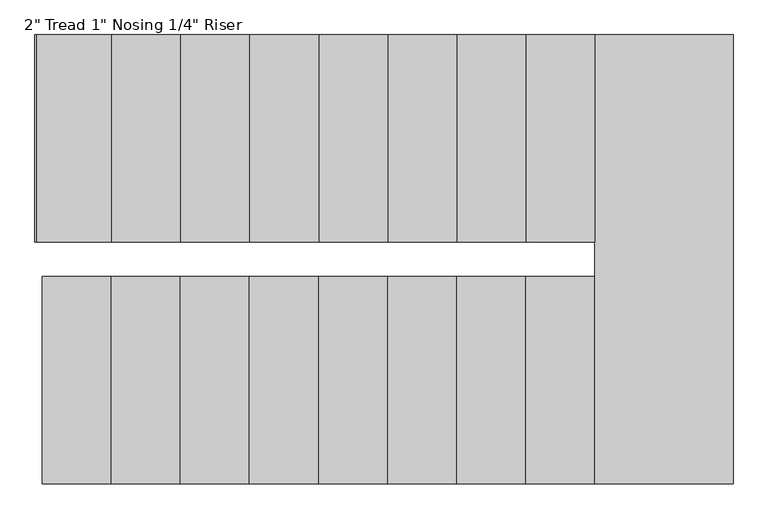
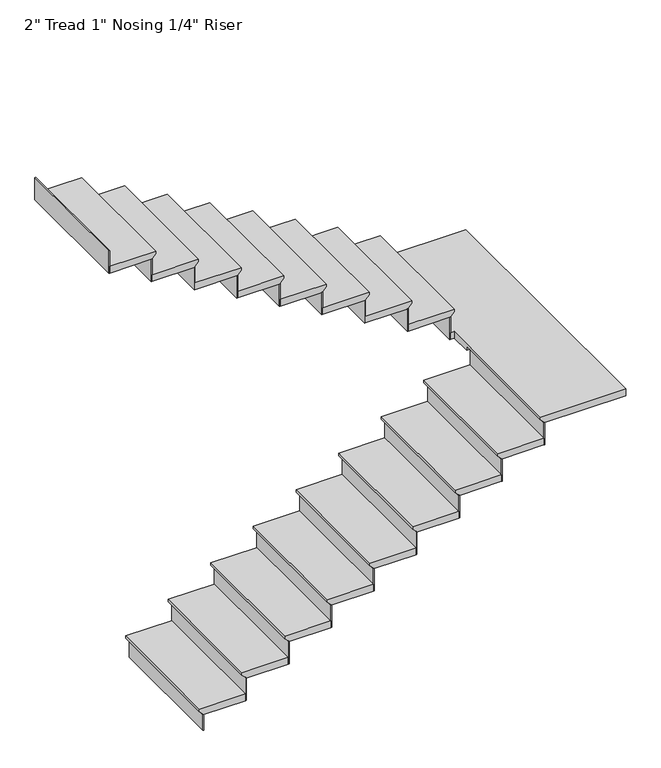
"""IFC4 building model written with IfcOpenShell, lengths in millimetres: stair flight geometry."""

from ifc_helpers import new_model, si_unit, origin, place, context, project, spatial, faceted_brep, source, transform, mapped, element, save


def stair_flight_ebc403c3(model_context):
    return source(origin(), model_context, "Body", "Brep", [
        faceted_brep([(-1197.97188, -4816.50869, 9599.0833333), (-1197.97188, -4816.50869, 9618.1333333), (-1197.97188, -3902.10869, 9618.1333333), (-1197.97188, -3902.10869, 9599.0833333), (-1172.57188, -4816.50869, 9573.6833333), (-1172.57188, -3902.10869, 9573.6833333), (-867.77188, -4816.50869, 9618.1333333), (-867.77188, -3902.10869, 9618.1333333), (-1172.57188, -3902.10869, 9567.3333333), (-867.77188, -3902.10869, 9567.3333333), (-867.77188, -4816.50869, 9567.3333333), (-1172.57188, -4816.50869, 9567.3333333)], [[[0, 1, 2, 3]], [[4, 0, 3, 5]], [[2, 1, 6, 7]], [[8, 9, 10, 11]], [[2, 7, 9, 8, 5, 3]], [[8, 11, 4, 5]], [[6, 1, 0, 4, 11, 10]], [[7, 6, 10, 9]]]),
        faceted_brep([(-1172.57188, -4816.50869, 9567.3333333), (-1172.57188, -4816.50869, 9448.8), (-1166.22188, -4816.50869, 9448.8), (-1166.22188, -4816.50869, 9567.3333333), (-1172.57188, -3902.10869, 9567.3333333), (-1166.22188, -3902.10869, 9567.3333333), (-1166.22188, -3902.10869, 9448.8), (-1172.57188, -3902.10869, 9448.8)], [[[0, 1, 2, 3]], [[4, 5, 6, 7]], [[1, 0, 4, 7]], [[2, 1, 7, 6]], [[3, 2, 6, 5]], [[0, 3, 5, 4]]]),
        faceted_brep([(-867.77188, -4816.50869, 9736.6666667), (-867.77188, -4816.50869, 9567.3333333), (-861.42188, -4816.50869, 9567.3333333), (-861.42188, -4816.50869, 9736.6666667), (-867.77188, -3902.10869, 9736.6666667), (-861.42188, -3902.10869, 9736.6666667), (-861.42188, -3902.10869, 9567.3333333), (-867.77188, -3902.10869, 9567.3333333)], [[[0, 1, 2, 3]], [[4, 5, 6, 7]], [[1, 0, 4, 7]], [[2, 1, 7, 6]], [[3, 2, 6, 5]], [[0, 3, 5, 4]]]),
        faceted_brep([(-893.17188, -3902.10869, 9787.4666667), (-893.17188, -4816.50869, 9787.4666667), (-562.97188, -4816.50869, 9787.4666667), (-562.97188, -3902.10869, 9787.4666667), (-867.77188, -3902.10869, 9736.6666667), (-562.97188, -3902.10869, 9736.6666667), (-562.97188, -4816.50869, 9736.6666667), (-867.77188, -4816.50869, 9736.6666667), (-867.77188, -3902.10869, 9743.0166667), (-893.17188, -3902.10869, 9768.4166667), (-867.77188, -4816.50869, 9743.0166667), (-893.17188, -4816.50869, 9768.4166667)], [[[0, 1, 2, 3]], [[4, 5, 6, 7]], [[0, 3, 5, 4, 8, 9]], [[4, 7, 10, 8]], [[2, 1, 11, 10, 7, 6]], [[3, 2, 6, 5]], [[11, 1, 0, 9]], [[10, 11, 9, 8]]]),
        faceted_brep([(-562.97188, -4816.50869, 9906.0), (-562.97188, -4816.50869, 9736.6666667), (-556.62188, -4816.50869, 9736.6666667), (-556.62188, -4816.50869, 9906.0), (-562.97188, -3902.10869, 9906.0), (-556.62188, -3902.10869, 9906.0), (-556.62188, -3902.10869, 9736.6666667), (-562.97188, -3902.10869, 9736.6666667)], [[[0, 1, 2, 3]], [[4, 5, 6, 7]], [[1, 0, 4, 7]], [[2, 1, 7, 6]], [[3, 2, 6, 5]], [[0, 3, 5, 4]]]),
        faceted_brep([(-588.37188, -3902.10869, 9956.8), (-588.37188, -4816.50869, 9956.8), (-258.17188, -4816.50869, 9956.8), (-258.17188, -3902.10869, 9956.8), (-562.97188, -3902.10869, 9906.0), (-258.17188, -3902.10869, 9906.0), (-258.17188, -4816.50869, 9906.0), (-562.97188, -4816.50869, 9906.0), (-562.97188, -3902.10869, 9912.35), (-588.37188, -3902.10869, 9937.75), (-562.97188, -4816.50869, 9912.35), (-588.37188, -4816.50869, 9937.75)], [[[0, 1, 2, 3]], [[4, 5, 6, 7]], [[0, 3, 5, 4, 8, 9]], [[4, 7, 10, 8]], [[2, 1, 11, 10, 7, 6]], [[3, 2, 6, 5]], [[11, 1, 0, 9]], [[10, 11, 9, 8]]]),
        faceted_brep([(-258.17188, -4816.50869, 10075.3333333), (-258.17188, -4816.50869, 9906.0), (-251.82188, -4816.50869, 9906.0), (-251.82188, -4816.50869, 10075.3333333), (-258.17188, -3902.10869, 10075.3333333), (-251.82188, -3902.10869, 10075.3333333), (-251.82188, -3902.10869, 9906.0), (-258.17188, -3902.10869, 9906.0)], [[[0, 1, 2, 3]], [[4, 5, 6, 7]], [[1, 0, 4, 7]], [[2, 1, 7, 6]], [[3, 2, 6, 5]], [[0, 3, 5, 4]]]),
        faceted_brep([(-283.57188, -3902.10869, 10126.1333333), (-283.57188, -4816.50869, 10126.1333333), (46.62812, -4816.50869, 10126.1333333), (46.62812, -3902.10869, 10126.1333333), (-258.17188, -3902.10869, 10075.3333333), (46.62812, -3902.10869, 10075.3333333), (46.62812, -4816.50869, 10075.3333333), (-258.17188, -4816.50869, 10075.3333333), (-258.17188, -3902.10869, 10081.6833333), (-283.57188, -3902.10869, 10107.0833333), (-258.17188, -4816.50869, 10081.6833333), (-283.57188, -4816.50869, 10107.0833333)], [[[0, 1, 2, 3]], [[4, 5, 6, 7]], [[0, 3, 5, 4, 8, 9]], [[4, 7, 10, 8]], [[2, 1, 11, 10, 7, 6]], [[3, 2, 6, 5]], [[11, 1, 0, 9]], [[10, 11, 9, 8]]]),
        faceted_brep([(46.62812, -4816.50869, 10244.6666667), (46.62812, -4816.50869, 10075.3333333), (52.97812, -4816.50869, 10075.3333333), (52.97812, -4816.50869, 10244.6666667), (46.62812, -3902.10869, 10244.6666667), (52.97812, -3902.10869, 10244.6666667), (52.97812, -3902.10869, 10075.3333333), (46.62812, -3902.10869, 10075.3333333)], [[[0, 1, 2, 3]], [[4, 5, 6, 7]], [[1, 0, 4, 7]], [[2, 1, 7, 6]], [[3, 2, 6, 5]], [[0, 3, 5, 4]]]),
        faceted_brep([(21.22812, -3902.10869, 10295.4666667), (21.22812, -4816.50869, 10295.4666667), (351.42812, -4816.50869, 10295.4666667), (351.42812, -3902.10869, 10295.4666667), (46.62812, -3902.10869, 10244.6666667), (351.42812, -3902.10869, 10244.6666667), (351.42812, -4816.50869, 10244.6666667), (46.62812, -4816.50869, 10244.6666667), (46.62812, -3902.10869, 10251.0166667), (21.22812, -3902.10869, 10276.4166667), (46.62812, -4816.50869, 10251.0166667), (21.22812, -4816.50869, 10276.4166667)], [[[0, 1, 2, 3]], [[4, 5, 6, 7]], [[0, 3, 5, 4, 8, 9]], [[4, 7, 10, 8]], [[2, 1, 11, 10, 7, 6]], [[3, 2, 6, 5]], [[11, 1, 0, 9]], [[10, 11, 9, 8]]]),
        faceted_brep([(351.42812, -4816.50869, 10414.0), (351.42812, -4816.50869, 10244.6666667), (357.77812, -4816.50869, 10244.6666667), (357.77812, -4816.50869, 10414.0), (351.42812, -3902.10869, 10414.0), (357.77812, -3902.10869, 10414.0), (357.77812, -3902.10869, 10244.6666667), (351.42812, -3902.10869, 10244.6666667)], [[[0, 1, 2, 3]], [[4, 5, 6, 7]], [[1, 0, 4, 7]], [[2, 1, 7, 6]], [[3, 2, 6, 5]], [[0, 3, 5, 4]]]),
        faceted_brep([(326.02812, -3902.10869, 10464.8), (326.02812, -4816.50869, 10464.8), (656.22812, -4816.50869, 10464.8), (656.22812, -3902.10869, 10464.8), (351.42812, -3902.10869, 10414.0), (656.22812, -3902.10869, 10414.0), (656.22812, -4816.50869, 10414.0), (351.42812, -4816.50869, 10414.0), (351.42812, -3902.10869, 10420.35), (326.02812, -3902.10869, 10445.75), (351.42812, -4816.50869, 10420.35), (326.02812, -4816.50869, 10445.75)], [[[0, 1, 2, 3]], [[4, 5, 6, 7]], [[0, 3, 5, 4, 8, 9]], [[4, 7, 10, 8]], [[2, 1, 11, 10, 7, 6]], [[3, 2, 6, 5]], [[11, 1, 0, 9]], [[10, 11, 9, 8]]]),
        faceted_brep([(656.22812, -4816.50869, 10583.3333333), (656.22812, -4816.50869, 10414.0), (662.57812, -4816.50869, 10414.0), (662.57812, -4816.50869, 10583.3333333), (656.22812, -3902.10869, 10583.3333333), (662.57812, -3902.10869, 10583.3333333), (662.57812, -3902.10869, 10414.0), (656.22812, -3902.10869, 10414.0)], [[[0, 1, 2, 3]], [[4, 5, 6, 7]], [[1, 0, 4, 7]], [[2, 1, 7, 6]], [[3, 2, 6, 5]], [[0, 3, 5, 4]]]),
        faceted_brep([(630.82812, -3902.10869, 10634.1333333), (630.82812, -4816.50869, 10634.1333333), (961.02812, -4816.50869, 10634.1333333), (961.02812, -3902.10869, 10634.1333333), (656.22812, -3902.10869, 10583.3333333), (961.02812, -3902.10869, 10583.3333333), (961.02812, -4816.50869, 10583.3333333), (656.22812, -4816.50869, 10583.3333333), (656.22812, -3902.10869, 10589.6833333), (630.82812, -3902.10869, 10615.0833333), (656.22812, -4816.50869, 10589.6833333), (630.82812, -4816.50869, 10615.0833333)], [[[0, 1, 2, 3]], [[4, 5, 6, 7]], [[0, 3, 5, 4, 8, 9]], [[4, 7, 10, 8]], [[2, 1, 11, 10, 7, 6]], [[3, 2, 6, 5]], [[11, 1, 0, 9]], [[10, 11, 9, 8]]]),
        faceted_brep([(961.02812, -4816.50869, 10752.6666667), (961.02812, -4816.50869, 10583.3333333), (967.37812, -4816.50869, 10583.3333333), (967.37812, -4816.50869, 10752.6666667), (961.02812, -3902.10869, 10752.6666667), (967.37812, -3902.10869, 10752.6666667), (967.37812, -3902.10869, 10583.3333333), (961.02812, -3902.10869, 10583.3333333)], [[[0, 1, 2, 3]], [[4, 5, 6, 7]], [[1, 0, 4, 7]], [[2, 1, 7, 6]], [[3, 2, 6, 5]], [[0, 3, 5, 4]]]),
        faceted_brep([(935.62812, -3902.10869, 10803.4666667), (935.62812, -4816.50869, 10803.4666667), (1265.82812, -4816.50869, 10803.4666667), (1265.82812, -3902.10869, 10803.4666667), (961.02812, -3902.10869, 10752.6666667), (1265.82812, -3902.10869, 10752.6666667), (1265.82812, -4816.50869, 10752.6666667), (961.02812, -4816.50869, 10752.6666667), (961.02812, -3902.10869, 10759.0166667), (935.62812, -3902.10869, 10784.4166667), (961.02812, -4816.50869, 10759.0166667), (935.62812, -4816.50869, 10784.4166667)], [[[0, 1, 2, 3]], [[4, 5, 6, 7]], [[0, 3, 5, 4, 8, 9]], [[4, 7, 10, 8]], [[2, 1, 11, 10, 7, 6]], [[3, 2, 6, 5]], [[11, 1, 0, 9]], [[10, 11, 9, 8]]]),
        faceted_brep([(1265.82812, -4816.50869, 10922.0), (1265.82812, -4816.50869, 10752.6666667), (1272.17812, -4816.50869, 10752.6666667), (1272.17812, -4816.50869, 10922.0), (1265.82812, -3902.10869, 10922.0), (1272.17812, -3902.10869, 10922.0), (1272.17812, -3902.10869, 10752.6666667), (1265.82812, -3902.10869, 10752.6666667)], [[[0, 1, 2, 3]], [[4, 5, 6, 7]], [[1, 0, 4, 7]], [[2, 1, 7, 6]], [[3, 2, 6, 5]], [[0, 3, 5, 4]]]),
        faceted_brep([(1215.02812, -3749.70869, 10972.8), (1240.42812, -3749.70869, 10972.8), (1240.42812, -4816.50869, 10972.8), (1850.02812, -4816.50869, 10972.8), (1850.02812, -2835.30869, 10972.8), (1215.02812, -2835.30869, 10972.8), (1240.42812, -3749.70869, 10922.0), (1215.02812, -3749.70869, 10922.0), (1215.02812, -2835.30869, 10922.0), (1850.02812, -2835.30869, 10922.0), (1850.02812, -4816.50869, 10922.0), (1265.82812, -4816.50869, 10922.0), (1265.82812, -3902.10869, 10922.0), (1240.42812, -3902.10869, 10922.0), (1240.42812, -3902.10869, 10953.75), (1240.42812, -4816.50869, 10953.75), (1265.82812, -3902.10869, 10928.35), (1265.82812, -4816.50869, 10928.35)], [[[0, 1, 2, 3, 4, 5]], [[6, 7, 8, 9, 10, 11, 12, 13]], [[1, 0, 7, 6]], [[2, 1, 6, 13, 14, 15]], [[13, 12, 16, 14]], [[12, 11, 17, 16]], [[3, 2, 15, 17, 11, 10]], [[4, 3, 10, 9]], [[5, 4, 9, 8]], [[0, 5, 8, 7]], [[17, 15, 14, 16]]]),
        faceted_brep([(1215.02812, -2835.30869, 11091.3333333), (1215.02812, -2835.30869, 10922.0), (1208.67812, -2835.30869, 10922.0), (1208.67812, -2835.30869, 11091.3333333), (1215.02812, -3749.70869, 11091.3333333), (1208.67812, -3749.70869, 11091.3333333), (1208.67812, -3749.70869, 10922.0), (1215.02812, -3749.70869, 10922.0)], [[[0, 1, 2, 3]], [[4, 5, 6, 7]], [[1, 0, 4, 7]], [[2, 1, 7, 6]], [[3, 2, 6, 5]], [[0, 3, 5, 4]]]),
        faceted_brep([(1240.42812, -3749.70869, 11142.1333333), (1240.42812, -2835.30869, 11142.1333333), (910.22812, -2835.30869, 11142.1333333), (910.22812, -3749.70869, 11142.1333333), (1215.02812, -3749.70869, 11091.3333333), (910.22812, -3749.70869, 11091.3333333), (910.22812, -2835.30869, 11091.3333333), (1215.02812, -2835.30869, 11091.3333333), (1215.02812, -3749.70869, 11097.6833333), (1240.42812, -3749.70869, 11123.0833333), (1215.02812, -2835.30869, 11097.6833333), (1240.42812, -2835.30869, 11123.0833333)], [[[0, 1, 2, 3]], [[4, 5, 6, 7]], [[0, 3, 5, 4, 8, 9]], [[4, 7, 10, 8]], [[2, 1, 11, 10, 7, 6]], [[3, 2, 6, 5]], [[11, 1, 0, 9]], [[10, 11, 9, 8]]]),
        faceted_brep([(910.22812, -2835.30869, 11260.6666667), (910.22812, -2835.30869, 11091.3333333), (903.87812, -2835.30869, 11091.3333333), (903.87812, -2835.30869, 11260.6666667), (910.22812, -3749.70869, 11260.6666667), (903.87812, -3749.70869, 11260.6666667), (903.87812, -3749.70869, 11091.3333333), (910.22812, -3749.70869, 11091.3333333)], [[[0, 1, 2, 3]], [[4, 5, 6, 7]], [[1, 0, 4, 7]], [[2, 1, 7, 6]], [[3, 2, 6, 5]], [[0, 3, 5, 4]]]),
        faceted_brep([(935.62812, -3749.70869, 11311.4666667), (935.62812, -2835.30869, 11311.4666667), (605.42812, -2835.30869, 11311.4666667), (605.42812, -3749.70869, 11311.4666667), (910.22812, -3749.70869, 11260.6666667), (605.42812, -3749.70869, 11260.6666667), (605.42812, -2835.30869, 11260.6666667), (910.22812, -2835.30869, 11260.6666667), (910.22812, -3749.70869, 11267.0166667), (935.62812, -3749.70869, 11292.4166667), (910.22812, -2835.30869, 11267.0166667), (935.62812, -2835.30869, 11292.4166667)], [[[0, 1, 2, 3]], [[4, 5, 6, 7]], [[0, 3, 5, 4, 8, 9]], [[4, 7, 10, 8]], [[2, 1, 11, 10, 7, 6]], [[3, 2, 6, 5]], [[11, 1, 0, 9]], [[10, 11, 9, 8]]]),
        faceted_brep([(605.42812, -2835.30869, 11430.0), (605.42812, -2835.30869, 11260.6666667), (599.07812, -2835.30869, 11260.6666667), (599.07812, -2835.30869, 11430.0), (605.42812, -3749.70869, 11430.0), (599.07812, -3749.70869, 11430.0), (599.07812, -3749.70869, 11260.6666667), (605.42812, -3749.70869, 11260.6666667)], [[[0, 1, 2, 3]], [[4, 5, 6, 7]], [[1, 0, 4, 7]], [[2, 1, 7, 6]], [[3, 2, 6, 5]], [[0, 3, 5, 4]]]),
        faceted_brep([(630.82812, -3749.70869, 11480.8), (630.82812, -2835.30869, 11480.8), (300.62812, -2835.30869, 11480.8), (300.62812, -3749.70869, 11480.8), (605.42812, -3749.70869, 11430.0), (300.62812, -3749.70869, 11430.0), (300.62812, -2835.30869, 11430.0), (605.42812, -2835.30869, 11430.0), (605.42812, -3749.70869, 11436.35), (630.82812, -3749.70869, 11461.75), (605.42812, -2835.30869, 11436.35), (630.82812, -2835.30869, 11461.75)], [[[0, 1, 2, 3]], [[4, 5, 6, 7]], [[0, 3, 5, 4, 8, 9]], [[4, 7, 10, 8]], [[2, 1, 11, 10, 7, 6]], [[3, 2, 6, 5]], [[11, 1, 0, 9]], [[10, 11, 9, 8]]]),
        faceted_brep([(300.62812, -2835.30869, 11599.3333333), (300.62812, -2835.30869, 11430.0), (294.27812, -2835.30869, 11430.0), (294.27812, -2835.30869, 11599.3333333), (300.62812, -3749.70869, 11599.3333333), (294.27812, -3749.70869, 11599.3333333), (294.27812, -3749.70869, 11430.0), (300.62812, -3749.70869, 11430.0)], [[[0, 1, 2, 3]], [[4, 5, 6, 7]], [[1, 0, 4, 7]], [[2, 1, 7, 6]], [[3, 2, 6, 5]], [[0, 3, 5, 4]]]),
        faceted_brep([(326.02812, -3749.70869, 11650.1333333), (326.02812, -2835.30869, 11650.1333333), (-4.17188, -2835.30869, 11650.1333333), (-4.17188, -3749.70869, 11650.1333333), (300.62812, -3749.70869, 11599.3333333), (-4.17188, -3749.70869, 11599.3333333), (-4.17188, -2835.30869, 11599.3333333), (300.62812, -2835.30869, 11599.3333333), (300.62812, -3749.70869, 11605.6833333), (326.02812, -3749.70869, 11631.0833333), (300.62812, -2835.30869, 11605.6833333), (326.02812, -2835.30869, 11631.0833333)], [[[0, 1, 2, 3]], [[4, 5, 6, 7]], [[0, 3, 5, 4, 8, 9]], [[4, 7, 10, 8]], [[2, 1, 11, 10, 7, 6]], [[3, 2, 6, 5]], [[11, 1, 0, 9]], [[10, 11, 9, 8]]]),
        faceted_brep([(-4.17188, -2835.30869, 11768.6666667), (-4.17188, -2835.30869, 11599.3333333), (-10.52188, -2835.30869, 11599.3333333), (-10.52188, -2835.30869, 11768.6666667), (-4.17188, -3749.70869, 11768.6666667), (-10.52188, -3749.70869, 11768.6666667), (-10.52188, -3749.70869, 11599.3333333), (-4.17188, -3749.70869, 11599.3333333)], [[[0, 1, 2, 3]], [[4, 5, 6, 7]], [[1, 0, 4, 7]], [[2, 1, 7, 6]], [[3, 2, 6, 5]], [[0, 3, 5, 4]]]),
        faceted_brep([(21.22812, -3749.70869, 11819.4666667), (21.22812, -2835.30869, 11819.4666667), (-308.97188, -2835.30869, 11819.4666667), (-308.97188, -3749.70869, 11819.4666667), (-4.17188, -3749.70869, 11768.6666667), (-308.97188, -3749.70869, 11768.6666667), (-308.97188, -2835.30869, 11768.6666667), (-4.17188, -2835.30869, 11768.6666667), (-4.17188, -3749.70869, 11775.0166667), (21.22812, -3749.70869, 11800.4166667), (-4.17188, -2835.30869, 11775.0166667), (21.22812, -2835.30869, 11800.4166667)], [[[0, 1, 2, 3]], [[4, 5, 6, 7]], [[0, 3, 5, 4, 8, 9]], [[4, 7, 10, 8]], [[2, 1, 11, 10, 7, 6]], [[3, 2, 6, 5]], [[11, 1, 0, 9]], [[10, 11, 9, 8]]]),
        faceted_brep([(-308.97188, -2835.30869, 11938.0), (-308.97188, -2835.30869, 11768.6666667), (-315.32188, -2835.30869, 11768.6666667), (-315.32188, -2835.30869, 11938.0), (-308.97188, -3749.70869, 11938.0), (-315.32188, -3749.70869, 11938.0), (-315.32188, -3749.70869, 11768.6666667), (-308.97188, -3749.70869, 11768.6666667)], [[[0, 1, 2, 3]], [[4, 5, 6, 7]], [[1, 0, 4, 7]], [[2, 1, 7, 6]], [[3, 2, 6, 5]], [[0, 3, 5, 4]]]),
        faceted_brep([(-283.57188, -3749.70869, 11988.8), (-283.57188, -2835.30869, 11988.8), (-613.77188, -2835.30869, 11988.8), (-613.77188, -3749.70869, 11988.8), (-308.97188, -3749.70869, 11938.0), (-613.77188, -3749.70869, 11938.0), (-613.77188, -2835.30869, 11938.0), (-308.97188, -2835.30869, 11938.0), (-308.97188, -3749.70869, 11944.35), (-283.57188, -3749.70869, 11969.75), (-308.97188, -2835.30869, 11944.35), (-283.57188, -2835.30869, 11969.75)], [[[0, 1, 2, 3]], [[4, 5, 6, 7]], [[0, 3, 5, 4, 8, 9]], [[4, 7, 10, 8]], [[2, 1, 11, 10, 7, 6]], [[3, 2, 6, 5]], [[11, 1, 0, 9]], [[10, 11, 9, 8]]]),
        faceted_brep([(-613.77188, -2835.30869, 12107.3333333), (-613.77188, -2835.30869, 11938.0), (-620.12188, -2835.30869, 11938.0), (-620.12188, -2835.30869, 12107.3333333), (-613.77188, -3749.70869, 12107.3333333), (-620.12188, -3749.70869, 12107.3333333), (-620.12188, -3749.70869, 11938.0), (-613.77188, -3749.70869, 11938.0)], [[[0, 1, 2, 3]], [[4, 5, 6, 7]], [[1, 0, 4, 7]], [[2, 1, 7, 6]], [[3, 2, 6, 5]], [[0, 3, 5, 4]]]),
        faceted_brep([(-588.37188, -3749.70869, 12158.1333333), (-588.37188, -2835.30869, 12158.1333333), (-918.57188, -2835.30869, 12158.1333333), (-918.57188, -3749.70869, 12158.1333333), (-613.77188, -3749.70869, 12107.3333333), (-918.57188, -3749.70869, 12107.3333333), (-918.57188, -2835.30869, 12107.3333333), (-613.77188, -2835.30869, 12107.3333333), (-613.77188, -3749.70869, 12113.6833333), (-588.37188, -3749.70869, 12139.0833333), (-613.77188, -2835.30869, 12113.6833333), (-588.37188, -2835.30869, 12139.0833333)], [[[0, 1, 2, 3]], [[4, 5, 6, 7]], [[0, 3, 5, 4, 8, 9]], [[4, 7, 10, 8]], [[2, 1, 11, 10, 7, 6]], [[3, 2, 6, 5]], [[11, 1, 0, 9]], [[10, 11, 9, 8]]]),
        faceted_brep([(-918.57188, -2835.30869, 12276.6666667), (-918.57188, -2835.30869, 12107.3333333), (-924.92188, -2835.30869, 12107.3333333), (-924.92188, -2835.30869, 12276.6666667), (-918.57188, -3749.70869, 12276.6666667), (-924.92188, -3749.70869, 12276.6666667), (-924.92188, -3749.70869, 12107.3333333), (-918.57188, -3749.70869, 12107.3333333)], [[[0, 1, 2, 3]], [[4, 5, 6, 7]], [[1, 0, 4, 7]], [[2, 1, 7, 6]], [[3, 2, 6, 5]], [[0, 3, 5, 4]]]),
        faceted_brep([(-1223.37188, -2835.30869, 12446.0), (-1223.37188, -2835.30869, 12276.6666667), (-1229.72188, -2835.30869, 12276.6666667), (-1229.72188, -2835.30869, 12446.0), (-1223.37188, -3749.70869, 12446.0), (-1229.72188, -3749.70869, 12446.0), (-1229.72188, -3749.70869, 12276.6666667), (-1223.37188, -3749.70869, 12276.6666667)], [[[0, 1, 2, 3]], [[4, 5, 6, 7]], [[1, 0, 4, 7]], [[2, 1, 7, 6]], [[3, 2, 6, 5]], [[0, 3, 5, 4]]]),
        faceted_brep([(-893.17188, -3749.70869, 12327.4666667), (-893.17188, -2835.30869, 12327.4666667), (-1223.37188, -2835.30869, 12327.4666667), (-1223.37188, -3749.70869, 12327.4666667), (-918.57188, -3749.70869, 12276.6666667), (-1223.37188, -3749.70869, 12276.6666667), (-1223.37188, -2835.30869, 12276.6666667), (-918.57188, -2835.30869, 12276.6666667), (-918.57188, -3749.70869, 12283.0166667), (-893.17188, -3749.70869, 12308.4166667), (-918.57188, -2835.30869, 12283.0166667), (-893.17188, -2835.30869, 12308.4166667)], [[[0, 1, 2, 3]], [[4, 5, 6, 7]], [[0, 3, 5, 4, 8, 9]], [[4, 7, 10, 8]], [[2, 1, 11, 10, 7, 6]], [[3, 2, 6, 5]], [[11, 1, 0, 9]], [[10, 11, 9, 8]]]),
    ])


if __name__ == "__main__":
    model = new_model("IFC4")
    model_context = context("Model", 3, world=origin())
    ifc_project = project(units=[si_unit("LENGTHUNIT", "METRE", prefix="MILLI")], contexts=[model_context])
    site = spatial("IfcSite", under=ifc_project)
    building = spatial("IfcBuilding", under=site)
    placement = place(None, origin())
    stair_flight_shape = stair_flight_ebc403c3(model_context)
    element("IfcStairFlight", 1, ObjectType="2\" Tread 1\" Nosing 1/4\" Riser", at=placement, inside=building, context=model_context, shape_type="MappedRepresentation", body=[
        mapped(stair_flight_shape, transform((0.0, 0.0, 0.0), x_axis=(1.0, 0.0, 0.0), y_axis=(0.0, 1.0, 0.0), z_axis=(0.0, 0.0, 1.0))),
    ])
    save(model, "model.ifc")
